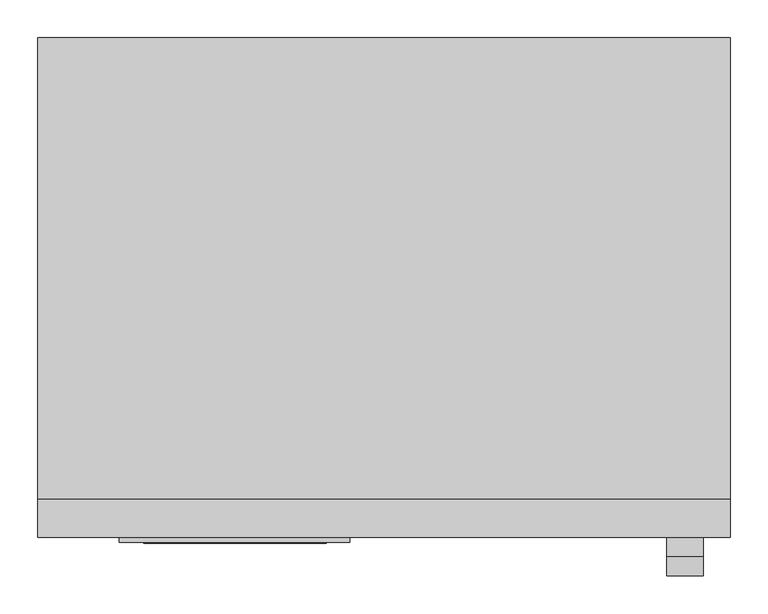
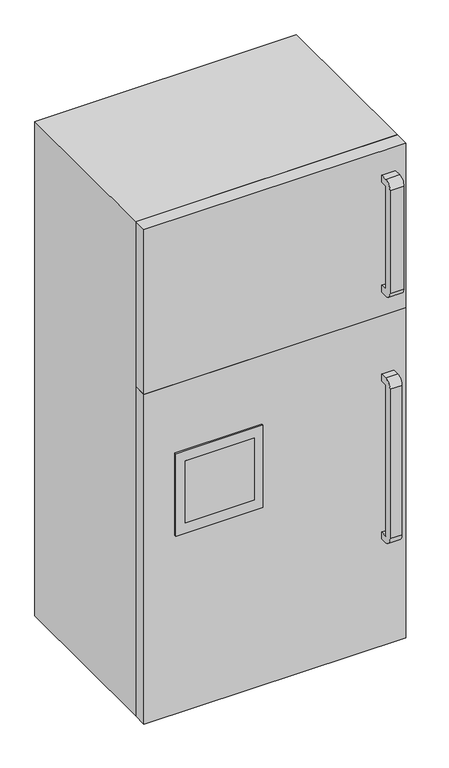
"""IFC4 building model written with IfcOpenShell, lengths in millimetres: furniture geometry."""

from ifc_helpers import new_model, si_unit, point, frame, frame_2d, origin, origin_with_axes, place, context, project, spatial, polyline, circle_curve, trimmed, segment, composite_curve, outline, extrude, faceted_brep, source, transform, mapped, element, save


def furniture_65fa61b5(model_context):
    return source(origin(), model_context, "Body", "SolidModel", [
        faceted_brep([(-154.8604727, -609.6, 0.0), (-154.8604727, -609.6, 1828.8), (-1069.2604727, -609.6, 1828.8), (-1069.2604727, -609.6, 0.0), (-983.107199, -609.6, 1745.9088241), (-221.107199, -609.6, 1745.9088241), (-221.107199, -609.6, 1288.7088241), (-983.107199, -609.6, 1288.7088241), (-983.107199, -609.6, 1168.6818903), (-221.107199, -609.6, 1168.6818903), (-221.107199, -609.6, 101.8818903), (-983.107199, -609.6, 101.8818903), (-154.8604727, 0.0, 0.0), (-1069.2604727, 0.0, 0.0), (-1069.2604727, 0.0, 1828.8), (-154.8604727, 0.0, 1828.8), (-221.107199, -101.6, 1745.9088241), (-983.107199, -101.6, 1745.9088241), (-983.107199, -101.6, 1288.7088241), (-221.107199, -101.6, 1288.7088241), (-221.107199, -101.6, 1168.6818903), (-983.107199, -101.6, 1168.6818903), (-983.107199, -101.6, 101.8818903), (-221.107199, -101.6, 101.8818903)], [[[0, 1, 2, 3], [4, 5, 6, 7], [8, 9, 10, 11]], [[12, 13, 14, 15]], [[1, 0, 12, 15]], [[2, 1, 15, 14]], [[3, 2, 14, 13]], [[0, 3, 13, 12]], [[16, 17, 18, 19]], [[17, 16, 5, 4]], [[18, 17, 4, 7]], [[19, 18, 7, 6]], [[16, 19, 6, 5]], [[20, 21, 22, 23]], [[21, 20, 9, 8]], [[22, 21, 8, 11]], [[23, 22, 11, 10]], [[20, 23, 10, 9]]]),
        extrude(outline(polyline([(-154.8604727, -660.4), (-1069.2604727, -660.4), (-1069.2604727, -609.6), (-154.8604727, -609.6), (-154.8604727, -660.4)])), frame((0.0, 0.0, 1220.3738546), z_axis=(0.0, 0.0, 1.0), x_axis=(1.0, 0.0, 0.0)), (0.0, 0.0, 1.0), 608.4261454),
        extrude(outline(polyline([(-154.8604727, -660.4), (-1069.2604727, -660.4), (-1069.2604727, -609.6), (-154.8604727, -609.6), (-154.8604727, -660.4)])), origin_with_axes(), (0.0, 0.0, 1.0), 1220.3738546),
        extrude(outline(composite_curve([segment(polyline([(-685.8, 1004.4738546), (-660.4, 1004.4738546), (-660.4, 979.0738546), (-685.8, 979.0738546), (-685.8, 420.2738546), (-660.4, 420.2738546), (-660.4, 394.8738546), (-679.45, 394.8738546)]), True, "CONTINUOUS"), segment(trimmed(circle_curve(frame_2d((-679.45, 426.6238546)), 31.75), [point((-679.45, 394.8738546))], [point((-711.2, 426.6238546))], False, "CARTESIAN"), True, "CONTINUOUS"), segment(polyline([(-711.2, 426.6238546), (-711.2, 979.0738546)]), True, "CONTINUOUS"), segment(trimmed(circle_curve(frame_2d((-685.8, 979.0738546)), 25.4), [point((-711.2, 979.0738546))], [point((-685.8, 1004.4738546))], False, "CARTESIAN"), True, "CONTINUOUS")], self_intersect=False)), frame((-238.6131994, 0.0, 0.0), z_axis=(1.0, 0.0, 0.0), x_axis=(0.0, 1.0, 0.0)), (0.0, 0.0, 1.0), 41.7631994),
        extrude(outline(composite_curve([segment(polyline([(-685.8, 1739.5588241), (-660.4, 1739.5588241), (-660.4, 1714.1588241), (-685.8, 1714.1588241), (-685.8, 1333.1588241), (-660.4, 1333.1588241), (-660.4, 1307.7588241), (-685.8, 1307.7588241)]), True, "CONTINUOUS"), segment(trimmed(circle_curve(frame_2d((-685.8, 1333.1588241)), 25.4), [point((-685.8, 1307.7588241))], [point((-711.2, 1333.1588241))], False, "CARTESIAN"), True, "CONTINUOUS"), segment(polyline([(-711.2, 1333.1588241), (-711.2, 1714.1588241)]), True, "CONTINUOUS"), segment(trimmed(circle_curve(frame_2d((-685.8, 1714.1588241)), 25.4), [point((-711.2, 1714.1588241))], [point((-685.8, 1739.5588241))], False, "CARTESIAN"), True, "CONTINUOUS")], self_intersect=False)), frame((-238.6131994, 0.0, 0.0), z_axis=(1.0, 0.0, 0.0), x_axis=(0.0, 1.0, 0.0)), (0.0, 0.0, 1.0), 48.1131994),
        extrude(outline(polyline([(-657.1290221, -666.75), (-961.9290221, -666.75), (-961.9290221, -609.6), (-657.1290221, -609.6), (-657.1290221, -666.75)])), frame((0.0, 0.0, 661.4796579), z_axis=(0.0, 0.0, 1.0), x_axis=(1.0, 0.0, 0.0)), (0.0, 0.0, 1.0), 304.8),
        extrude(outline(polyline([(-688.2162761, -668.3375), (-929.5162761, -668.3375), (-929.5162761, -648.467525), (-688.2162761, -648.467525), (-688.2162761, -668.3375)])), frame((0.0, 0.0, 700.7556373), z_axis=(0.0, 0.0, 1.0), x_axis=(1.0, 0.0, 0.0)), (0.0, 0.0, 1.0), 228.6),
    ])


if __name__ == "__main__":
    model = new_model("IFC4")
    model_context = context("Model", 3, world=origin())
    ifc_project = project(units=[si_unit("LENGTHUNIT", "METRE", prefix="MILLI")], contexts=[model_context])
    site = spatial("IfcSite", under=ifc_project)
    building = spatial("IfcBuilding", under=site)
    placement = place(None, origin())
    furniture_shape = furniture_65fa61b5(model_context)
    element("IfcFurniture", 1, at=placement, inside=building, context=model_context, shape_type="MappedRepresentation", body=[
        mapped(furniture_shape, transform((0.0, 0.0, 0.0), x_axis=(1.0, 0.0, 0.0), y_axis=(0.0, 1.0, 0.0), z_axis=(0.0, 0.0, 1.0))),
    ])
    save(model, "model.ifc")

# Revit data of these elements
# Type
#   Default Elevation = 0
# Element 1 (IfcFurniture)
#   Materials on its faces: "Default", "Default 3", "Default 2"
# Materials
#   "Default": colour RGB 127 127 127, transparency 0, Cost = 0
#   "Default 3": class "Glass", colour RGB 127 127 127, transparency 0
#   "Default 2": class "Plastic", colour RGB 127 127 127, transparency 0
